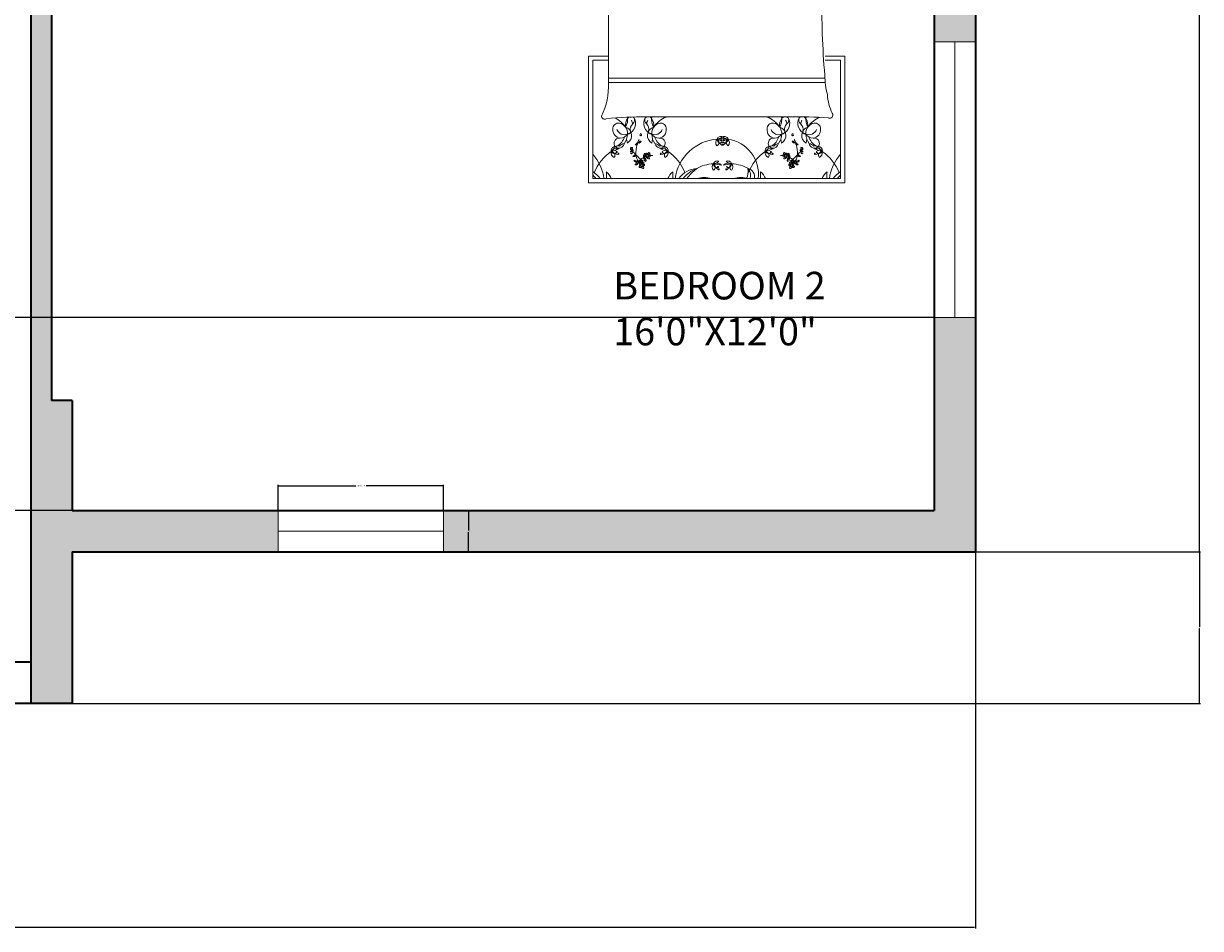
# Model space of a CAD drawing. Units: inches. Extents: x -26 to 13070, y -956 to 6917.
# Tile 3 of 13: x 341 to 597, y -956 to -760. Entities that reach past the tile are written whole.
import ezdxf

# ---------------------------------------------------------------- set-up
doc = ezdxf.new("R2010")
doc.units = ezdxf.units.IN
doc.header["$MEASUREMENT"] = 0
for name, color, linetype, lineweight in [('A-ANNO-DIMS', 2, 'Continuous', 18), ('A-AREA-IDEN', 7, 'Continuous', 18), ('A-FURN', 8, 'Continuous', 13), ('A-GLAZ', 4, 'Continuous', 18), ('A-WALL', 7, 'Continuous', 35), ('A-WALL-PATT', 252, 'Continuous', 13)]:
    doc.layers.add(name, color=color, linetype=linetype, lineweight=lineweight)
doc.styles.get("Standard").update_dxf_attribs({"font": 'arial.ttf'})
doc.dimstyles.get("Standard").update_dxf_attribs({"dimtxt": 0.18, "dimasz": 0.18, "dimexe": 0.18, "dimexo": 0.0625, "dimgap": 0.09, "dimtad": 0, "dimtih": 1, "dimtoh": 1, "dimdec": 0, "dimzin": 0, "dimdsep": 46, "dimlunit": 3, "dimtxsty": 'Standard', "dimcen": 0.09, "dimadec": 0, "dimazin": 0, "dimtfac": 1, "dimtdec": 0, "dimtofl": 0, "dimtmove": 0, "dimatfit": 3, "dimfxl": 1, "dimtolj": 1, "dimtzin": 0, "dimarcsym": 0})

# ---------------------------------------------------------------- blocks, each defined once
blk = doc.blocks.new('BED-DOUBLE-NIGHTSTANDS')
for p, q in [((0, 65), (76.43, 65)), ((15.29, 65), (15.29, 44.02)), ((61.14, 64.02), (15.29, 64.02)), ((7.64, 53.64), (7.64, 63.62)), ((68.79, 53.64), (68.79, 63.62)), ((12.64, 58.63), (2.65, 58.63)), ((63.79, 58.63), (73.78, 58.63)), ((15.29, 52.92), (61.14, 52.92)), ((25.9, 50.65), (34.24, 52.92)), ((36.28, 52.92), (32.09, 47.09)), ((20.33, 48.64), (25.9, 50.65)), ((60.91, 48.96), (33.16, 48.57)), ((60.94, 49.74), (33.73, 49.36)), ((14.6, 43.22), (17.39, 46.47)), ((17.39, 46.47), (20.33, 48.64)), ((32.09, 47.09), (30.39, 42.6)), ((60.87, 46.55), (31.85, 46.44)), ((60.87, 45.77), (31.55, 45.65)), ((15.22, 42.6), (14.6, 43.22)), ((18.32, 42.91), (15.22, 42.6)), ((22.19, 42.6), (18.32, 42.91)), ((25.59, 42.14), (22.19, 42.6)), ((27.6, 41.21), (25.59, 42.14)), ((30.08, 40.59), (27.6, 41.21)), ((30.39, 42.6), (30.08, 40.59)), ((10.09, 27.53), (14.41, 27.53)), ((10.09, 0), (10.09, 27.53)), ((14.41, 26.65), (10.97, 26.65)), ((10.97, 26.65), (10.97, 0.89)), ((64.92, 26.65), (61.55, 26.65)), ((61.57, 27.53), (65.81, 27.53)), ((64.92, 0.89), (64.92, 26.65)), ((65.81, 27.53), (65.81, 0)), ((61.56, 21.81), (14.4, 21.81)), ((61.49, 22.77), (14.41, 22.77)), ((53.73, 14.3), (22.7, 14.3)), ((18.51, 8.63), (18.34, 9.5)), ((23.85, 8.63), (24.02, 9.5)), ((52.05, 8.63), (51.88, 9.5)), ((57.39, 8.63), (57.56, 9.5)), ((10.97, 0.89), (64.92, 0.89)), ((65.81, 0), (10.09, 0))]:
    blk.add_line(p, q)
for points in [[(15.29, 52.26), (0, 52.26), (0, 65)], [(61.14, 65), (61.14, 52.26), (76.43, 52.26), (76.43, 65)], [(7.64, 58.63), (8.53, 60.17)], [(68.79, 58.63), (67.89, 60.17)], [(7.64, 58.63), (8.53, 57.08)], [(68.79, 58.63), (67.89, 57.08)]]:
    blk.add_lwpolyline(points)
for points in [[(19.68, 63.09, 0.074897), (19.77, 58.1, -0.472817)], [(37.86, 57.82, 0.14099), (38.01, 62.91, 0.235245)], [(41.12, 57.82, -0.14099), (40.97, 62.91, -0.235245)], [(56.75, 63.09, -0.074897), (56.66, 58.1, 0.472817)], [(14.44, 36.22, 0.001242), (14.4, 21.72, -0.127202), (12.87, 14.5)], [(61.47, 23.37, 0.056112), (62.02, 19.16, 0.095341), (63.1, 15.11)]]:
    blk.add_lwpolyline(points, format="xyb")
for centre, radius in [((7.64, 58.63), 3.57), ((68.79, 58.63), 3.57), ((7.64, 58.63), 1.78), ((68.79, 58.63), 1.78), ((22.92, 5.86), 0.195), ((52.98, 5.86), 0.195), ((21.65, 3.81), 0.195), ((54.25, 3.81), 0.195)]:
    blk.add_circle(centre, radius)
for centre, radius, start, end in [((61.8, 790.45), 728.57, 266.68521, 267.14978), ((30.15, 35.44), 27.72, 82.2196, 99.497), ((36, 49.44), 13.62, 81.5249, 103.96), ((42.02, 59.28), 3.78, 63.3437, 106.1026), ((47.68, 49.72), 13.44, 76.3427, 101.1841), ((14.63, 790.45), 728.57, 272.85022, 273.31479), ((29.41, 56.1), 9.85, 155.1316, 191.7583), ((47.02, 56.1), 9.85, 348.2417, 24.8684), ((28.85, 55.27), 9.36, 354.0129, 15.8293), ((50.13, 55.27), 9.36, 164.1707, 185.9871), ((22.4, 63.99), 10.24, 255.1039, 281.0369), ((27.79, 71.27), 17.76, 258.0397, 289.2615), ((34.99, 67.39), 13.48, 259.8617, 283.6238), ((42.53, 57.96), 4.05, 245.0183, 288.5407), ((49.61, 63.23), 9.73, 243.8761, 286.1746), ((54.03, 63.99), 10.24, 258.9631, 284.8961), ((198.16, 43.58), 137.33, 176.1, 180.9282), ((-55.48, 41.32), 70.1, 355.8294, 1.553), ((15.91, 70.29), 28.85, 267.4519, 281.3392), ((22.8, 35.91), 6.22, 66.2616, 101.3392), ((35.39, 69.47), 29.64, 250.1194, 259.3383), ((239.96, 38.59), 179.14, 179.1145, 184.8735), ((29.91, 40.53), 0.184, 268.8623, 19.7536), ((13.58, 14.54), 0.705, 183.98, 297.3412), ((21.79, -65.25), 79.56, 89.3433, 95.6887), ((16.65, 11.7), 1.29, 84.4856, 181.0538), ((13.28, 8.92), 5.78, 33.6671, 63.2997), ((16.25, 10.75), 2.3, 355.2933, 76.921), ((21.03, 12.36), 2.95, 145.785, 184.7304), ((15.4, 13.74), 3.17, 328.8218, 9.1554), ((19.32, 13.46), 0.92, 120.0293, 142.325), ((17.85, 12.92), 2.44, 289.2822, 29.1751), ((17.48, 12.48), 2.2, 7.436, 29.9149), ((18.93, 13.64), 1.14, 311.5653, 23.8354), ((19.32, 13.46), 0.92, 44.4517, 63.558), ((24.5, 12.92), 2.44, 150.8249, 250.7178), ((23.42, 13.64), 1.14, 156.1646, 228.4347), ((23.03, 13.46), 0.92, 113.229, 135.5483), ((24.87, 12.48), 2.2, 150.0851, 172.564), ((23.03, 13.46), 0.92, 37.675, 66.7144), ((21.32, 12.36), 2.95, 355.2696, 34.215), ((26.95, 13.74), 3.17, 169.7133, 211.1782), ((26.1, 10.75), 2.3, 103.079, 184.7067), ((29.07, 8.92), 5.78, 111.4941, 146.3329), ((25.7, 11.7), 1.29, 358.9462, 95.5144), ((50.19, 11.7), 1.29, 84.4856, 181.0538), ((46.82, 8.92), 5.78, 33.6671, 68.5059), ((49.8, 10.75), 2.3, 355.2933, 76.921), ((54.57, 12.36), 2.95, 145.785, 184.7304), ((48.94, 13.74), 3.17, 328.8218, 10.2867), ((52.87, 13.46), 0.92, 113.2856, 142.325), ((51.4, 12.92), 2.44, 289.2822, 29.1751), ((51.03, 12.48), 2.2, 7.436, 29.9149), ((52.87, 13.46), 0.92, 44.4517, 66.7144), ((52.48, 13.64), 1.14, 311.5653, 23.8354), ((56.07, -60.03), 74.37, 85.2402, 91.8035), ((58.04, 12.92), 2.44, 150.8249, 250.7178), ((56.96, 13.64), 1.14, 156.1646, 228.4347), ((56.57, 13.46), 0.92, 106.6343, 135.5483), ((58.41, 12.48), 2.2, 150.0851, 172.564), ((56.57, 13.46), 0.92, 37.675, 72.5814), ((54.87, 12.36), 2.95, 355.2696, 34.215), ((60.5, 13.74), 3.17, 169.249, 211.1782), ((59.64, 10.75), 2.3, 103.079, 184.7067), ((62.62, 8.92), 5.78, 113.6453, 146.3329), ((59.25, 11.7), 1.29, 358.9462, 95.5144), ((62.52, 14.72), 0.697, 246.5219, 33.8264), ((17.18, 11.52), 1.83, 174.9449, 262.8857), ((17.9, 12.21), 1.77, 201.5819, 291.4221), ((16.86, 11.92), 2.22, 272.3591, 324.0401), ((14.45, 10.81), 4.1, 326.2883, 356.5076), ((17.56, 10.28), 1.9, 299.9085, 73.1337), ((21.03, 12.36), 2.95, 212.7011, 216.3445), ((18.76, 11.08), 0.474, 257.3041, 15.1471), ((20.73, 11.61), 1.57, 131.5653, 195.1471), ((21.4, 10.36), 0.147, 102.7051, 280.4384), ((21.38, 10.45), 0.24, 280.4384, 100.4136), ((21.62, 11.61), 1.57, 344.8529, 48.4347), ((24.79, 10.28), 1.9, 106.8663, 240.0915), ((23.59, 11.08), 0.474, 164.8529, 282.6959), ((21.32, 12.36), 2.95, 323.6555, 327.2989), ((25.49, 11.92), 2.22, 215.9599, 267.6409), ((24.46, 12.21), 1.77, 248.5779, 338.4181), ((27.9, 10.81), 4.1, 183.4924, 213.7117), ((25.17, 11.52), 1.83, 277.1143, 5.0551), ((50.72, 11.52), 1.83, 174.9449, 262.8857), ((51.44, 12.21), 1.77, 201.5819, 291.4221), ((50.4, 11.92), 2.22, 272.3591, 324.0401), ((47.99, 10.81), 4.1, 326.2883, 356.5076), ((51.1, 10.28), 1.9, 299.9085, 73.1337), ((54.57, 12.36), 2.95, 212.7011, 216.3445), ((52.3, 11.08), 0.474, 257.3041, 15.1471), ((54.28, 11.61), 1.57, 131.5653, 195.1471), ((54.52, 10.45), 0.24, 79.5864, 259.5616), ((54.5, 10.36), 0.147, 259.5616, 77.2949), ((55.16, 11.61), 1.57, 344.8529, 48.4347), ((58.34, 10.28), 1.9, 106.8663, 240.0915), ((57.13, 11.08), 0.474, 164.8529, 282.6959), ((54.87, 12.36), 2.95, 323.6555, 327.2989), ((59.04, 11.92), 2.22, 215.9599, 267.6409), ((58, 12.21), 1.77, 248.5779, 338.4181), ((61.45, 10.81), 4.1, 183.4924, 213.7117), ((58.72, 11.52), 1.83, 277.1143, 5.0551), ((15.79, 6.99), 0.827, 92.9516, 193.728), ((14.09, 8.25), 1.7, 301.3827, 345.2969), ((16.76, 8.57), 1.15, 80.264, 250.8688), ((16.52, 7.33), 0.703, 63.9755, 143.2681), ((14.48, 11.1), 3.61, 301.2614, 341.7045), ((16.48, 8.92), 1.43, 265.969, 344.3045), ((18.02, 7.01), 1.53, 96.1662, 141.5825), ((19.47, 7.55), 0.15, 345.2356, 144.9248), ((20.55, 8.08), 0.401, 101.3256, 154.4621), ((19.97, 9.45), 1.21, 280.2588, 300.656), ((20.25, 10.41), 2.16, 268.3264, 277.1302), ((26.69, 6.51), 6.33, 163.5842, 183.8277), ((19.71, 9.44), 1.23, 308.2101, 316.3071), ((20.47, 8.64), 0.367, 278.3432, 4.2869), ((20.26, 8.96), 0.641, 300.656, 332.6341), ((20.74, 8.53), 0.156, 55.7657, 157.4417), ((26.69, 6.51), 6.33, 153.0032, 159.8941), ((20.99, 8.68), 0.156, 84.3784, 186.0543), ((20.84, 9.3), 0.641, 269.1859, 301.164), ((21.03, 8.97), 0.367, 237.5332, 323.4768), ((20.67, 10.02), 1.23, 285.5129, 293.6099), ((20.55, 9.79), 1.21, 301.164, 321.5612), ((21.48, 8.64), 0.401, 87.3579, 140.4944), ((19.56, 10), 2.16, 324.6898, 333.4936), ((27.87, 11.1), 3.61, 198.2955, 238.7386), ((24.33, 7.01), 1.53, 38.4175, 83.8338), ((25.87, 8.92), 1.43, 195.6955, 274.031), ((25.59, 8.57), 1.15, 289.1312, 99.736), ((25.83, 7.33), 0.703, 36.7319, 116.0245), ((26.57, 6.99), 0.827, 346.272, 87.0484), ((28.26, 8.25), 1.7, 194.7031, 238.6173), ((38.81, -0.46), 9.98, 94.4623, 172.255), ((38.85, 8.75), 1.11, 137.7873, 219.1145), ((37.6, 8.78), 0.834, 298.5391, 58.3627), ((38.83, 9.26), 0.827, 63.0274, 163.8037), ((37.99, 11.2), 1.7, 271.4585, 315.3727), ((38.68, 8.05), 1.58, 45.5411, 114.3101), ((40.12, 16.15), 6.98, 252.593, 267.2582), ((38.85, 9.46), 0.816, 177.7585, 283.852), ((40.42, 10.31), 2.52, 198.9159, 238.011), ((39.76, 8.05), 1.58, 65.6899, 134.4589), ((38.32, 16.15), 6.98, 272.7418, 287.407), ((39.02, 8.77), 0.108, 283.852, 219.9245), ((39.15, 8.27), 0.124, 238.011, 71.5592), ((39.17, 8.33), 0.0602, 71.5592, 188.0167), ((39.29, 8.27), 0.124, 108.4408, 301.989), ((39.62, 9.26), 0.827, 16.1963, 116.9726), ((40.45, 11.2), 1.7, 224.6273, 268.5415), ((39.27, 8.33), 0.0602, 351.9833, 108.4408), ((39.42, 8.81), 0.0651, 320.1909, 256.0209), ((38.02, 10.31), 2.52, 301.989, 341.0841), ((39.6, 9.46), 0.816, 256.148, 2.2415), ((40.85, 8.78), 0.834, 121.6373, 241.4609), ((39.59, 8.75), 1.11, 320.8855, 42.2127), ((39.31, 1.85), 7.72, 352.8636, 81.8197), ((49.33, 6.99), 0.827, 92.9516, 193.728), ((47.64, 8.25), 1.7, 301.3827, 345.2969), ((50.3, 8.57), 1.15, 80.264, 250.8688), ((50.06, 7.33), 0.703, 63.9755, 143.2681), ((48.03, 11.1), 3.61, 301.2614, 341.7045), ((50.03, 8.92), 1.43, 265.969, 344.3045), ((51.57, 7.01), 1.53, 96.1662, 141.5825), ((55.35, 9.79), 1.21, 218.4388, 238.836), ((54.42, 8.64), 0.401, 39.5056, 92.6421), ((56.33, 10), 2.16, 206.5064, 215.3102), ((54.87, 8.97), 0.367, 216.5232, 302.4668), ((55.05, 9.3), 0.641, 238.836, 270.8141), ((55.22, 10.02), 1.23, 246.3901, 254.4871), ((49.2, 6.51), 6.33, 20.1059, 26.9968), ((54.91, 8.68), 0.156, 353.9457, 95.6216), ((55.15, 8.53), 0.156, 22.5583, 124.2343), ((55.43, 8.64), 0.367, 175.7131, 261.6568), ((55.63, 8.96), 0.641, 207.3659, 239.344), ((49.2, 6.51), 6.33, 356.1723, 16.4158), ((56.18, 9.44), 1.23, 223.6929, 231.7899), ((55.92, 9.45), 1.21, 239.344, 259.7412), ((55.64, 10.41), 2.16, 262.8698, 271.6736), ((55.34, 8.08), 0.401, 25.5379, 78.6744), ((56.42, 7.55), 0.15, 35.0752, 194.7644), ((61.41, 11.1), 3.61, 198.2955, 238.7386), ((59.41, 8.92), 1.43, 195.6955, 274.031), ((57.87, 7.01), 1.53, 38.4175, 83.8338), ((59.14, 8.57), 1.15, 289.1312, 99.736), ((59.37, 7.33), 0.703, 36.7319, 116.0245), ((61.8, 8.25), 1.7, 194.7031, 238.6173), ((60.11, 6.99), 0.827, 346.272, 87.0484), ((3.54, -0.46), 9.98, 7.745, 41.8856), ((20.62, -1.45), 9.98, 124.3865, 158.5908), ((16.06, 6.55), 1.11, 167.7115, 249.0387), ((16.26, 5.87), 1.58, 75.4653, 144.2343), ((13.47, 13.61), 6.98, 282.5173, 297.1824), ((14.96, 5.96), 0.834, 328.4633, 88.2869), ((16.64, 8.69), 2.52, 228.8402, 267.9352), ((15.7, 7.17), 0.816, 207.6827, 313.7762), ((16.19, 6.66), 0.108, 313.7762, 249.7183), ((16.54, 6.35), 0.0602, 101.4834, 217.9409), ((16.56, 6.29), 0.124, 267.9352, 101.4834), ((19.42, 7.32), 0.325, 101.5637, 142.6358), ((19.15, 7.02), 0.195, 273.2768, 86.7232), ((19.41, 6.66), 0.321, 217.7621, 259.0403), ((19.37, 7.21), 0.186, 91.1081, 181.8675), ((19.76, 7.09), 0.591, 203.4276, 227.6104), ((19.57, 6.83), 0.402, 80.3487, 133.6538), ((19.5, 7.16), 0.318, 229.7889, 317.6792), ((19.16, 7.58), 0.468, 288.7263, 352.5032), ((19.14, 6.49), 0.452, 355.053, 68.3618), ((19.5, 6.41), 0.637, 83.0852, 105.7171), ((19.44, 6.46), 0.149, 232.4737, 355.053), ((15.08, 1.13), 7.26, 43.1541, 52.0459), ((19.61, 7.06), 0.168, 317.6792, 80.3487), ((20.1, 5.51), 0.401, 101.3256, 154.4621), ((19.52, 6.87), 1.21, 280.2588, 300.656), ((19.8, 7.84), 2.16, 268.3264, 277.1302), ((19.26, 6.87), 1.23, 308.2101, 316.3071), ((20.01, 6.06), 0.367, 278.3432, 4.2869), ((19.81, 6.39), 0.641, 300.656, 332.6341), ((20.29, 5.96), 0.156, 55.7657, 157.4417), ((23.54, 6.35), 3.17, 184.756, 209.2041), ((28.11, 13.11), 10.44, 222.2412, 232.1744), ((23.87, 2.14), 3.81, 120.544, 139.818), ((21.43, 6.15), 0.887, 304.5369, 16.3699), ((21.9, 5.96), 0.539, 272.8499, 356.1226), ((21.52, 5.75), 0.522, 321.7607, 7.9252), ((21.63, 5), 0.522, 8.7227, 54.8872), ((21.66, 4.58), 0.887, 0.278, 72.111), ((22.66, 5.9), 0.628, 127.3105, 187.9252), ((22.06, 4.9), 0.539, 20.5253, 88.5375), ((21.8, 5.98), 0.645, 355.0106, 41.658), ((22.51, 5.5), 0.193, 148.0499, 225.6268), ((23.87, 2.14), 3.81, 113.0501, 113.8477), ((22.87, 5.28), 0.614, 104.7558, 148.0499), ((22.52, 5.72), 0.384, 247.4086, 351.4386), ((22.71, 6.14), 0.265, 126.1046, 271.4281), ((22.68, 6.21), 0.191, 353.7526, 131.7054), ((22.63, 5.7), 0.129, 262.906, 7.132), ((22.5, 5.98), 0.268, 0.0645, 61.1507), ((22.56, 6.21), 0.306, 311.8413, 355.7877), ((23.19, 5.5), 0.321, 151.2196, 259.0403), ((23.19, 6.17), 0.325, 101.5637, 176.365), ((23.15, 6.05), 0.186, 91.1081, 181.8675), ((23.53, 5.93), 0.591, 203.4276, 227.6104), ((23.35, 5.67), 0.402, 80.3487, 133.6538), ((23.27, 6.01), 0.318, 229.7889, 317.6792), ((22.93, 6.42), 0.468, 288.7263, 352.5032), ((22.91, 5.33), 0.452, 355.053, 68.3618), ((23.27, 5.26), 0.637, 83.0852, 105.7171), ((23.25, 6.4), 0.15, 345.2356, 144.9248), ((23.22, 5.31), 0.149, 232.4737, 355.053), ((23.38, 5.91), 0.168, 317.6792, 80.3487), ((23.87, 2.14), 3.81, 87.1071, 94.7585), ((25.8, 6.29), 0.124, 78.5166, 272.0648), ((26.09, 5.87), 1.58, 35.7657, 104.5347), ((28.88, 13.61), 6.98, 242.8176, 257.4827), ((25.71, 8.69), 2.52, 272.0648, 311.1598), ((25.81, 6.35), 0.0602, 322.0591, 78.5166), ((26.65, 7.17), 0.816, 226.2238, 332.3173), ((26.17, 6.7), 0.0651, 290.2667, 226.2271), ((27.4, 5.96), 0.834, 91.7131, 211.5367), ((26.29, 6.55), 1.11, 290.9613, 12.2885), ((21.73, -1.45), 9.98, 21.4092, 55.6135), ((54.16, -1.45), 9.98, 124.3865, 158.5908), ((49.61, 6.55), 1.11, 167.7115, 249.0387), ((49.81, 5.87), 1.58, 75.4653, 144.2343), ((47.01, 13.61), 6.98, 282.5173, 297.1824), ((49.25, 7.17), 0.816, 207.6827, 313.7762), ((50.19, 8.69), 2.52, 228.8402, 267.9352), ((48.5, 5.96), 0.834, 328.4633, 88.2869), ((49.74, 6.66), 0.108, 313.7762, 249.7183), ((50.09, 6.35), 0.0602, 101.4834, 217.9409), ((50.1, 6.29), 0.124, 267.9352, 101.4834), ((52.03, 2.14), 3.81, 85.2415, 92.8929), ((52.51, 5.91), 0.168, 99.6513, 222.3208), ((52.62, 6.01), 0.318, 222.3208, 310.2111), ((52.55, 5.67), 0.402, 46.3462, 99.6513), ((52.65, 6.4), 0.15, 35.0752, 194.7644), ((52.97, 6.42), 0.468, 187.4968, 251.2737), ((52.98, 5.33), 0.452, 111.6382, 184.947), ((52.68, 5.31), 0.149, 184.947, 307.5263), ((52.63, 5.26), 0.637, 74.2829, 96.9148), ((52.75, 6.05), 0.186, 358.1325, 88.8919), ((52.36, 5.93), 0.591, 312.3896, 336.5724), ((52.71, 6.17), 0.325, 3.635, 78.4363), ((52.71, 5.5), 0.321, 280.9597, 28.7804), ((53.37, 5.72), 0.384, 188.5614, 292.5914), ((53.22, 6.21), 0.191, 48.2946, 186.2474), ((53.34, 6.21), 0.306, 184.2123, 228.1587), ((53.4, 5.98), 0.268, 118.8493, 179.9355), ((53.26, 5.7), 0.129, 172.868, 277.094), ((53.19, 6.14), 0.265, 268.5719, 53.8954), ((53.03, 5.28), 0.614, 31.9501, 75.2442), ((53.84, 4.9), 0.539, 91.4625, 159.4747), ((54.23, 4.58), 0.887, 107.889, 179.722), ((54.1, 5.98), 0.645, 138.342, 184.9894), ((53.99, 5.96), 0.539, 183.8774, 267.1501), ((52.03, 2.14), 3.81, 66.1523, 66.9499), ((53.38, 5.5), 0.193, 314.3732, 31.9501), ((54.47, 6.15), 0.887, 163.6301, 235.4631), ((53.23, 5.9), 0.628, 352.0748, 52.6895), ((54.26, 5), 0.522, 125.1128, 171.2773), ((54.37, 5.75), 0.522, 172.0748, 218.2393), ((52.03, 2.14), 3.81, 40.182, 59.456), ((47.79, 13.11), 10.44, 307.8256, 317.7588), ((52.36, 6.35), 3.17, 330.7959, 355.244), ((60.81, 1.13), 7.26, 127.9541, 136.8459), ((55.61, 5.96), 0.156, 22.5583, 124.2343), ((55.88, 6.06), 0.367, 175.7131, 261.6568), ((56.09, 6.39), 0.641, 207.3659, 239.344), ((56.64, 6.87), 1.23, 223.6929, 231.7899), ((56.38, 6.87), 1.21, 239.344, 259.7412), ((56.1, 7.84), 2.16, 262.8698, 271.6736), ((55.8, 5.51), 0.401, 25.5379, 78.6744), ((56.28, 7.06), 0.168, 99.6513, 222.3208), ((56.4, 7.16), 0.318, 222.3208, 310.2111), ((56.32, 6.83), 0.402, 46.3462, 99.6513), ((56.74, 7.58), 0.468, 187.4968, 251.2737), ((56.76, 6.49), 0.452, 111.6382, 184.947), ((56.45, 6.46), 0.149, 184.947, 307.5263), ((56.4, 6.41), 0.637, 74.2829, 96.9148), ((56.52, 7.21), 0.186, 358.1325, 88.8919), ((56.14, 7.09), 0.591, 312.3896, 336.5724), ((56.48, 7.32), 0.325, 37.3642, 78.4363), ((56.48, 6.66), 0.321, 280.9597, 322.2379), ((56.75, 7.02), 0.195, 93.2768, 266.7232), ((59.34, 6.29), 0.124, 78.5166, 272.0648), ((59.63, 5.87), 1.58, 35.7657, 104.5347), ((62.43, 13.61), 6.98, 242.8176, 257.4827), ((59.25, 8.69), 2.52, 272.0648, 311.1598), ((59.35, 6.35), 0.0602, 322.0591, 78.5166), ((60.19, 7.17), 0.816, 226.2238, 332.3173), ((59.71, 6.7), 0.0651, 290.2667, 226.2271), ((60.94, 5.96), 0.834, 91.7131, 211.5367), ((59.83, 6.55), 1.11, 290.9613, 12.2885), ((55.28, -1.45), 9.98, 21.4092, 55.6135), ((72.35, -0.46), 9.98, 138.1144, 172.255), ((20.23, 4.81), 0.217, 146.8636, 236.9021), ((23.3, 9.6), 5.69, 235.1882, 238.8844), ((20.6, 5.12), 0.588, 199.4799, 267.6828), ((20.54, 4.9), 0.507, 212.8155, 277.3992), ((20.24, 4.56), 0.588, 266.9701, 338.2913), ((17.14, 8.76), 5.69, 302.6784, 306.3746), ((20.39, 4.1), 0.217, 214.3538, 304.3923), ((20.47, 4.92), 0.225, 238.8844, 314.2646), ((20.42, 4.42), 0.507, 280.3057, 17.1958), ((20.38, 4.36), 0.225, 306.3746, 21.7548), ((20.75, 4.51), 0.17, 19.3605, 201.7548), ((20.75, 4.64), 0.17, 311.8703, 134.2646), ((23.94, 3.09), 3.39, 153.7819, 158.2913), ((21.24, 5.41), 0.887, 247.2305, 319.0635), ((20.95, 5.11), 0.522, 264.4544, 310.6188), ((23.54, 6.35), 3.17, 214.0033, 222.4917), ((21.33, 4.9), 0.539, 218.3208, 298.8162), ((21.24, 3.45), 0.193, 148.0499, 225.6268), ((21.6, 3.23), 0.614, 104.7558, 148.0499), ((21.25, 3.66), 0.384, 247.4086, 351.4386), ((21.43, 4.08), 0.265, 126.1046, 271.4281), ((21.4, 4.16), 0.191, 353.7526, 131.7054), ((21.7, 4.23), 0.628, 70.0041, 130.6188), ((21.36, 3.65), 0.129, 262.906, 7.132), ((21.22, 3.93), 0.268, 0.0645, 61.1507), ((21.29, 4.16), 0.306, 311.8413, 355.7877), ((21.29, 5), 0.645, 297.7043, 344.3516), ((21.92, 4.11), 0.325, 101.5637, 176.365), ((21.91, 3.45), 0.321, 151.2196, 259.0403), ((21.87, 4), 0.186, 91.1081, 181.8675), ((22.26, 3.88), 0.591, 203.4276, 227.6104), ((22.07, 3.62), 0.402, 80.3487, 133.6538), ((22, 3.96), 0.318, 229.7889, 317.6792), ((21.66, 4.37), 0.468, 288.7263, 352.5032), ((21.64, 3.28), 0.452, 355.053, 68.3618), ((22, 3.21), 0.637, 83.0852, 105.7171), ((21.97, 4.35), 0.15, 345.2356, 144.9248), ((21.94, 3.26), 0.149, 232.4737, 355.053), ((22.11, 3.85), 0.168, 317.6792, 80.3487), ((22.77, 5.17), 0.628, 188.7227, 249.3375), ((21.96, 4.86), 0.645, 334.9899, 21.6373), ((33.8, -1.8), 4.86, 91.272, 146.5383), ((35.55, -2.7), 6.06, 107.8504, 143.6964), ((38.74, -4.41), 9.02, 124.0123, 144.053), ((38.04, -5.81), 9.98, 94.4623, 117.4146), ((38.09, 3.4), 1.11, 137.7873, 219.1145), ((36.83, 3.44), 0.834, 298.5391, 58.3627), ((38.06, 3.91), 0.827, 63.0274, 163.8037), ((37.22, 5.85), 1.7, 271.4585, 315.3727), ((37.92, 2.71), 1.58, 45.5411, 114.3101), ((39.66, 4.96), 2.52, 198.9159, 238.011), ((39.36, 10.81), 6.98, 252.593, 267.2582), ((38.08, 4.11), 0.816, 177.7585, 283.852), ((38.25, 3.43), 0.108, 283.852, 219.9245), ((38.38, 2.93), 0.124, 238.011, 71.5592), ((38.4, 2.99), 0.0602, 71.5592, 188.0167), ((40.53, 2.71), 1.58, 65.6899, 134.4589), ((39.09, 10.81), 6.98, 272.7418, 287.407), ((40.06, 2.93), 0.124, 108.4408, 301.989), ((40.38, 3.91), 0.827, 16.1963, 116.9726), ((41.22, 5.85), 1.7, 224.6273, 268.5415), ((40.04, 2.99), 0.0602, 351.9833, 108.4408), ((40.18, 3.47), 0.0651, 320.1909, 256.0209), ((38.79, 4.96), 2.52, 301.989, 341.0841), ((40.36, 4.11), 0.816, 256.148, 2.2415), ((41.61, 3.44), 0.834, 121.6373, 241.4609), ((40.36, 3.4), 1.11, 320.8855, 42.2127), ((40.4, -5.81), 9.98, 62.5854, 85.5377), ((40.31, 2.55), 4.47, 338.117, 6.6195), ((44.41, 1.31), 1.79, 346.3898, 79.0739), ((43.06, 1.55), 2.27, 342.8609, 41.9049), ((53.93, 4.86), 0.645, 158.3627, 205.0101), ((53.13, 5.17), 0.628, 290.6625, 351.2773), ((53.78, 3.85), 0.168, 99.6513, 222.3208), ((53.9, 3.96), 0.318, 222.3208, 310.2111), ((53.82, 3.62), 0.402, 46.3462, 99.6513), ((53.92, 4.35), 0.15, 35.0752, 194.7644), ((54.24, 4.37), 0.468, 187.4968, 251.2737), ((54.26, 3.28), 0.452, 111.6382, 184.947), ((53.95, 3.26), 0.149, 184.947, 307.5263), ((53.9, 3.21), 0.637, 74.2829, 96.9148), ((54.2, 4.23), 0.628, 49.3812, 109.9959), ((54.65, 5.41), 0.887, 220.9365, 292.7695), ((54.6, 5), 0.645, 195.6484, 242.2957), ((54.02, 4), 0.186, 358.1325, 88.8919), ((53.64, 3.88), 0.591, 312.3896, 336.5724), ((53.98, 4.11), 0.325, 3.635, 78.4363), ((53.98, 3.45), 0.321, 280.9597, 28.7804), ((54.64, 3.66), 0.384, 188.5614, 292.5914), ((54.56, 4.9), 0.539, 241.1838, 321.6792), ((54.49, 4.16), 0.191, 48.2946, 186.2474), ((54.61, 4.16), 0.306, 184.2123, 228.1587), ((54.67, 3.93), 0.268, 118.8493, 179.9355), ((54.54, 3.65), 0.129, 172.868, 277.094), ((54.46, 4.08), 0.265, 268.5719, 53.8954), ((54.3, 3.23), 0.614, 31.9501, 75.2442), ((54.95, 5.11), 0.522, 229.3812, 275.5456), ((52.36, 6.35), 3.17, 317.5083, 325.9967), ((54.66, 3.45), 0.193, 314.3732, 31.9501), ((55.47, 4.42), 0.507, 162.8042, 259.6943), ((55.15, 4.64), 0.17, 45.7354, 228.1297), ((55.15, 4.51), 0.17, 338.2452, 160.6395), ((51.96, 3.09), 3.39, 21.7087, 26.2181), ((55.65, 4.56), 0.588, 201.7087, 273.0299), ((55.42, 4.92), 0.225, 225.7354, 301.1156), ((55.36, 4.9), 0.507, 262.6008, 327.1845), ((55.51, 4.36), 0.225, 158.2452, 233.6254), ((55.29, 5.12), 0.588, 272.3172, 340.5201), ((58.75, 8.76), 5.69, 233.6254, 237.3216), ((55.5, 4.1), 0.217, 235.6077, 325.6462), ((52.6, 9.6), 5.69, 301.1156, 304.8118), ((55.66, 4.81), 0.217, 303.0979, 33.1364), ((8.55, -1.8), 4.86, 33.4617, 60.1116), ((6.8, -2.7), 6.06, 36.3036, 46.4814), ((11.27, -0.67), 4.06, 22.5547, 48.9546), ((0.16, 1.51), 13.81, 357.4081, 3.6519), ((31.08, -0.67), 4.06, 131.0454, 157.4453), ((42.19, 1.51), 13.81, 176.3481, 182.5919), ((35.25, -4.36), 5.49, 73.5431, 107.0202), ((37.43, -7.19), 8.12, 94.3787, 95.6357), ((41.7, -12.75), 14.5, 109.7217, 109.9028), ((43.19, -4.36), 5.49, 72.9798, 106.4569), ((41.02, -7.19), 8.12, 84.3643, 85.6213), ((36.74, -12.75), 14.5, 70.0972, 70.2783), ((33.7, 1.51), 13.81, 357.4081, 3.6519), ((44.82, -0.67), 4.06, 22.5547, 48.9546), ((64.62, -0.67), 4.06, 131.0454, 157.4453), ((75.74, 1.51), 13.81, 176.3481, 182.5919), ((67.35, -1.8), 4.86, 119.8884, 146.5383), ((69.1, -2.7), 6.06, 133.5186, 143.6964)]:
    blk.add_arc(centre, radius, start, end)
blk = doc.blocks.new('WIN-36')
for p, q in [((0, 36), (0, 0)), ((9, 36), (0, 36)), ((4.5, 36), (4.5, 0)), ((9, 0), (9, 36)), ((0, 0), (9, 0))]:
    blk.add_line(p, q)
blk = doc.blocks.new('WIN-60')
for p, q in [((0, 0), (0, 60)), ((0, 60), (9, 60)), ((4.5, 0), (4.5, 60)), ((9, 60), (9, 0)), ((9, 0), (0, 0))]:
    blk.add_line(p, q)
blk = doc.blocks.new('*D18')
at = {"layer": 'A-ANNO-DIMS', "color": 0, "lineweight": -2, "transparency": 16777216}
for p, q in [((395.95, -865.48), (395.95, -859.96)), ((396.13, -860.14), (412.83, -860.14)), ((431.77, -860.14), (415.07, -860.14)), ((431.95, -865.48), (431.95, -859.96))]:
    blk.add_line(p, q, dxfattribs=at)
at = {"layer": 'A-ANNO-DIMS', "color": 0, "transparency": 16777216}
for points in [[(396.13, -860.11), (396.13, -860.17), (395.95, -860.14)], [(431.77, -860.11), (431.77, -860.17), (431.95, -860.14)]]:
    blk.add_solid(points, dxfattribs=at)
at = {"layer": 'Defpoints', "color": 0, "transparency": 16777216}
for p in [(395.95, -860.14), (395.95, -865.54), (431.95, -865.54)]:
    blk.add_point(p, dxfattribs=at)
at = {"layer": 'A-ANNO-DIMS', "color": 0, "transparency": 16777216, "insert": (413.95, -860.14), "char_height": 0.18, "attachment_point": 5}
blk.add_mtext('\\A1;WINDOW 36 TYP.', dxfattribs=at)
blk = doc.blocks.new('*D19')
at = {"layer": 'A-ANNO-DIMS', "color": 0, "lineweight": -2, "transparency": 16777216}
for p, q in [((432.01, -865.54), (437.53, -865.54)), ((437.35, -865.72), (437.35, -869.86)), ((437.35, -874.36), (437.35, -870.22)), ((432.01, -874.54), (437.53, -874.54))]:
    blk.add_line(p, q, dxfattribs=at)
at = {"layer": 'A-ANNO-DIMS', "color": 0, "transparency": 16777216}
for points in [[(437.32, -865.72), (437.38, -865.72), (437.35, -865.54)], [(437.32, -874.36), (437.38, -874.36), (437.35, -874.54)]]:
    blk.add_solid(points, dxfattribs=at)
at = {"layer": 'Defpoints', "color": 0, "transparency": 16777216}
for p in [(431.95, -865.54), (437.35, -865.54), (431.95, -874.54)]:
    blk.add_point(p, dxfattribs=at)
at = {"layer": 'A-ANNO-DIMS', "color": 0, "transparency": 16777216, "insert": (437.35, -870.04), "char_height": 0.18, "attachment_point": 5}
blk.add_mtext('\\A1;9 TYP.', dxfattribs=at)
blk = doc.blocks.new('*D40')
at = {"layer": 'A-ANNO-DIMS', "color": 0, "lineweight": -2, "transparency": 16777216}
for p, q in [((22.64, -874.6), (22.64, -956.47)), ((547.64, -874.6), (547.64, -956.47)), ((22.82, -956.29), (284.85, -956.29)), ((547.46, -956.29), (285.43, -956.29))]:
    blk.add_line(p, q, dxfattribs=at)
at = {"layer": 'A-ANNO-DIMS', "color": 0, "transparency": 16777216}
for points in [[(22.82, -956.26), (22.82, -956.32), (22.64, -956.29)], [(547.46, -956.26), (547.46, -956.32), (547.64, -956.29)]]:
    blk.add_solid(points, dxfattribs=at)
at = {"layer": 'Defpoints', "color": 0, "transparency": 16777216}
for p in [(22.64, -874.54), (547.64, -874.54), (547.64, -956.29)]:
    blk.add_point(p, dxfattribs=at)
at = {"layer": 'A-ANNO-DIMS', "color": 0, "transparency": 16777216, "insert": (285.14, -956.29), "char_height": 0.18, "attachment_point": 5}
blk.add_mtext('\\A1;525', dxfattribs=at)
blk = doc.blocks.new('*D46')
at = {"layer": 'A-ANNO-DIMS', "color": 0, "lineweight": -2, "transparency": 16777216}
for p, q in [((538.7, -457.54), (596.57, -457.54)), ((596.39, -457.72), (596.39, -665.86)), ((596.39, -874.36), (596.39, -666.22)), ((547.7, -874.54), (596.57, -874.54))]:
    blk.add_line(p, q, dxfattribs=at)
at = {"layer": 'A-ANNO-DIMS', "color": 0, "transparency": 16777216}
for points in [[(596.36, -457.72), (596.42, -457.72), (596.39, -457.54)], [(596.36, -874.36), (596.42, -874.36), (596.39, -874.54)]]:
    blk.add_solid(points, dxfattribs=at)
at = {"layer": 'Defpoints', "color": 0, "transparency": 16777216}
for p in [(538.64, -457.54), (596.39, -457.54), (547.64, -874.54)]:
    blk.add_point(p, dxfattribs=at)
at = {"layer": 'A-ANNO-DIMS', "color": 0, "transparency": 16777216, "insert": (596.39, -666.04), "char_height": 0.18, "attachment_point": 5}
blk.add_mtext('\\A1;417', dxfattribs=at)
blk = doc.blocks.new('*D48')
at = {"layer": 'A-ANNO-DIMS', "color": 0, "lineweight": -2, "transparency": 16777216}
for p, q in [((547.7, -874.54), (596.57, -874.54)), ((596.39, -874.72), (596.39, -890.86)), ((596.39, -907.36), (596.39, -891.22)), ((351.2, -907.54), (596.57, -907.54))]:
    blk.add_line(p, q, dxfattribs=at)
at = {"layer": 'A-ANNO-DIMS', "color": 0, "transparency": 16777216}
for points in [[(596.36, -874.72), (596.42, -874.72), (596.39, -874.54)], [(596.36, -907.36), (596.42, -907.36), (596.39, -907.54)]]:
    blk.add_solid(points, dxfattribs=at)
at = {"layer": 'Defpoints', "color": 0, "transparency": 16777216}
for p in [(547.64, -874.54), (596.39, -874.54), (351.14, -907.54)]:
    blk.add_point(p, dxfattribs=at)
at = {"layer": 'A-ANNO-DIMS', "color": 0, "transparency": 16777216, "insert": (596.39, -891.04), "char_height": 0.18, "attachment_point": 5}
blk.add_mtext('\\A1;33', dxfattribs=at)
blk = doc.blocks.new('*D59')
at = {"layer": 'A-ANNO-DIMS', "color": 0, "lineweight": -2, "transparency": 16777216}
for p, q in [((538.58, -823.54), (-26.29, -823.54)), ((-26.11, -823.72), (-26.11, -844.36)), ((-26.11, -865.36), (-26.11, -844.72)), ((538.58, -865.54), (-26.29, -865.54))]:
    blk.add_line(p, q, dxfattribs=at)
at = {"layer": 'A-ANNO-DIMS', "color": 0, "transparency": 16777216}
for points in [[(-26.14, -823.72), (-26.08, -823.72), (-26.11, -823.54)], [(-26.14, -865.36), (-26.08, -865.36), (-26.11, -865.54)]]:
    blk.add_solid(points, dxfattribs=at)
at = {"layer": 'Defpoints', "color": 0, "transparency": 16777216}
for p in [(-26.11, -823.54), (538.64, -823.54), (538.64, -865.54)]:
    blk.add_point(p, dxfattribs=at)
at = {"layer": 'A-ANNO-DIMS', "color": 0, "transparency": 16777216, "insert": (-26.11, -844.54), "char_height": 0.18, "attachment_point": 5}
blk.add_mtext('\\A1;42', dxfattribs=at)

msp = doc.modelspace()

# ---------------------------------------------------------------- hatches: boundary and pattern name
at = {"layer": 'A-WALL-PATT'}
h = msp.add_hatch(color=256, dxfattribs=at)
h.dxf.hatch_style = 1
h.paths.add_polyline_path([(223.641, 10.458), (214.641, 10.458), (22.641, 10.458), (22.641, -171.042), (31.641, -171.042), (31.641, -135.042), (205.641, -135.042), (205.641, -241.042), (210.141, -241.042), (210.141, -130.542), (94.641, -130.542), (94.641, -76.542), (85.641, -76.542), (85.641, -126.042), (27.141, -126.042), (27.141, 5.958), (85.641, 5.958), (85.641, -52.542), (94.641, -52.542), (94.641, 1.458), (214.641, 1.458), (214.641, -16.542), (223.641, -16.542), (229.641, -16.542), (229.641, -7.542), (223.641, -7.542)])
h.paths.add_polyline_path([(367.048, 10.458), (346.641, 10.458), (337.641, 10.458), (337.641, -7.542), (331.641, -7.542), (331.641, -16.542), (337.641, -16.542), (342.141, -16.542), (342.141, -128.542), (346.641, -128.542), (346.641, 1.458), (367.048, 1.458)])
h.paths.add_polyline_path([(547.641, 10.458), (403.048, 10.458), (403.048, 1.458), (538.641, 1.458), (538.641, -46.542), (547.641, -46.542)])
h.paths.add_polyline_path([(547.641, -106.542), (538.641, -106.542), (538.641, -154.542), (481.013, -154.542), (481.013, -159.042), (538.641, -159.042), (547.641, -159.042)])
h.paths.add_polyline_path([(457.013, -154.542), (342.141, -154.542), (342.141, -165.042), (346.641, -165.042), (346.641, -159.042), (414.141, -159.042), (414.141, -225.042), (346.641, -225.042), (346.641, -189.042), (342.141, -189.042), (342.141, -234.042), (390.641, -234.042), (390.641, -286.042), (395.141, -286.042), (395.141, -234.042), (456.141, -234.042), (456.141, -312.042), (372.641, -312.042), (372.641, -316.542), (462.641, -316.542), (462.641, -312.042), (460.641, -312.042), (460.641, -234.042), (538.641, -234.042), (547.641, -234.042), (547.641, -195.042), (538.641, -195.042), (538.641, -225.042), (418.641, -225.042), (418.641, -159.042), (457.013, -159.042)])
h.paths.add_polyline_path([(547.641, -270.042), (538.641, -270.042), (538.641, -312.042), (486.641, -312.042), (486.641, -316.542), (538.641, -316.542), (547.641, -316.542)], flags=0)
h.paths.add_polyline_path([(547.641, -456.306), (538.641, -456.306), (538.641, -457.542), (346.641, -457.542), (346.641, -316.542), (346.641, -312.042), (342.141, -312.042), (342.141, -457.542), (145.641, -457.542), (145.641, -466.542), (342.141, -466.542), (342.141, -627.042), (346.641, -627.042), (346.641, -466.542), (538.641, -466.542), (538.641, -514.542), (547.641, -514.542)])
h.paths.add_polyline_path([(466.641, -622.542), (372.641, -622.542), (372.641, -627.042), (388.641, -627.042), (388.641, -721.542), (393.141, -721.542), (393.141, -627.042), (462.141, -627.042), (462.141, -717.042), (466.641, -717.042)])
h.paths.add_polyline_path([(547.641, -574.542), (538.641, -574.542), (538.641, -622.542), (492.641, -622.542), (492.641, -627.042), (538.641, -627.042), (538.641, -654.042), (547.641, -654.042)])
h.paths.add_polyline_path([(547.641, -690.042), (538.641, -690.042), (538.641, -717.042), (466.641, -717.042), (466.641, -721.542), (538.641, -721.542), (538.641, -763.542), (547.641, -763.542)])
h.paths.add_polyline_path([(462.141, -717.042), (419.141, -717.042), (419.141, -721.542), (462.141, -721.542)], flags=0)
h.paths.add_polyline_path([(346.641, -721.542), (352.641, -721.542), (352.641, -717.042), (342.141, -717.042), (342.141, -874.542), (342.141, -907.542), (351.141, -907.542), (351.141, -874.542), (395.949, -874.542), (395.949, -865.542), (351.141, -865.542), (351.141, -841.542), (346.641, -841.542)])
h.paths.add_polyline_path([(547.641, -823.542), (538.641, -823.542), (538.641, -865.542), (431.949, -865.542), (431.949, -874.542), (547.641, -874.542)])
h.paths.add_polyline_path([(172.641, -865.713), (140.641, -865.744), (140.641, -788.744), (182.646, -788.704), (182.641, -784.204), (136.141, -784.249), (136.141, -848.332), (131.641, -848.332), (131.641, -874.542), (172.641, -874.542)])
h.paths.add_polyline_path([(217.641, -816.13), (213.141, -816.13), (213.141, -784.174), (208.641, -784.179), (208.641, -865.679), (208.641, -874.542), (217.641, -874.542)])
h.paths.add_polyline_path([(95.641, -865.788), (31.641, -865.849), (31.641, -832.695), (22.641, -832.695), (22.641, -874.542), (95.641, -874.542)])
h.paths.add_polyline_path([(217.641, -741.17), (31.641, -741.349), (31.641, -708.349), (22.641, -708.349), (22.641, -772.542), (22.641, -796.695), (31.641, -796.695), (31.641, -763.542), (31.641, -745.849), (217.641, -745.67)])
h.paths.add_polyline_path([(31.641, -651.349), (99.65, -651.284), (99.641, -642.284), (31.641, -642.349), (31.641, -639.042), (31.641, -588.349), (125.641, -588.259), (125.641, -651.259), (134.641, -651.25), (134.641, -579.25), (112.641, -579.271), (112.641, -549.042), (112.641, -504.271), (85.633, -504.297), (85.641, -513.297), (103.641, -513.28), (103.641, -549.042), (103.641, -579.28), (31.641, -579.349), (31.641, -549.042), (31.641, -513.349), (49.641, -513.314), (49.633, -504.332), (31.641, -504.349), (22.641, -504.358), (22.641, -684.349), (31.641, -684.349)])
h.paths.add_polyline_path([(31.641, -276.042), (145.641, -276.042), (145.641, -402.042), (145.641, -419.542), (154.641, -419.542), (154.641, -411.042), (154.641, -271.542), (210.141, -271.542), (210.141, -265.042), (205.641, -265.042), (205.641, -267.042), (31.641, -267.042), (31.641, -231.042), (22.641, -231.042), (22.641, -426.852), (31.641, -426.852), (31.641, -411.042), (31.641, -402.042)])

# ---------------------------------------------------------------- linework, layer by layer
at = {"layer": 'A-WALL'}
for p, q in [((547.641, 10.458), (547.641, -874.542)), ((342.141, -717.042), (342.141, -874.542)), ((346.641, -721.542), (346.641, -841.542)), ((538.641, -721.542), (538.641, -865.542)), ((351.141, -841.542), (346.641, -841.542)), ((351.141, -841.542), (351.141, -865.542)), ((351.141, -865.542), (538.641, -865.542)), ((342.141, -874.542), (342.141, -907.542)), ((351.141, -874.542), (351.141, -907.542)), ((351.141, -874.542), (547.641, -874.542)), ((342.141, -898.542), (222.141, -898.542)), ((351.141, -907.542), (222.141, -907.542))]:
    msp.add_line(p, q, dxfattribs=at)

# ---------------------------------------------------------------- block references
at = {"layer": 'A-FURN'}
msp.add_blockref('BED-DOUBLE-NIGHTSTANDS', (453.402, -794.181), dxfattribs=at)
at = {"layer": 'A-GLAZ'}
msp.add_blockref('WIN-60', (538.641, -823.542), dxfattribs=at)
at = {"layer": 'A-GLAZ', "rotation": 90}
msp.add_blockref('WIN-36', (431.948, -874.542), dxfattribs=at)

# ---------------------------------------------------------------- texts
at = {"layer": 'A-AREA-IDEN', "insert": (468.868, -813.577), "char_height": 6, "attachment_point": 1}
msp.add_mtext('BEDROOM 2\\P16\'0"X12\'0"', dxfattribs=at)

# ---------------------------------------------------------------- dimensions: what is measured, and where the dimension line sits
at = {"layer": 'A-ANNO-DIMS'}
for base, p1, p2, picture, middle in [((596.392, -457.542), (547.641, -874.542), (538.641, -457.542), '*D46', (596.392, -666.042)), ((-26.11, -823.542), (538.641, -865.542), (538.641, -823.542), '*D59', (-26.11, -844.542)), ((596.392, -874.542), (351.141, -907.542), (547.641, -874.542), '*D48', (596.392, -891.042))]:
    dim = msp.add_linear_dim(base=base, p1=p1, p2=p2, angle=90, dimstyle='Standard', override={"dimdec": 0, "dimlfac": 1, "dimrnd": 0, "dimzin": 0, "dimdsep": 46, "dimlunit": 2}, dxfattribs=at)
    dim.commit()
    dim.dimension.update_dxf_attribs({"geometry": picture, "text_midpoint": middle})
for base, p1, p2, angle, text, picture, middle in [((395.949, -860.142), (431.949, -865.542), (395.949, -865.542), 180, 'WINDOW <> TYP.', '*D18', (413.949, -860.142)), ((437.349, -865.542), (431.949, -874.542), (431.949, -865.542), 90, '<> TYP.', '*D19', (437.349, -870.042))]:
    dim = msp.add_linear_dim(base=base, p1=p1, p2=p2, angle=angle, text=text, dimstyle='Standard', override={"dimdec": 0, "dimlfac": 1, "dimrnd": 0, "dimzin": 0, "dimdsep": 46, "dimlunit": 2}, dxfattribs=at)
    dim.commit()
    dim.dimension.update_dxf_attribs({"geometry": picture, "text_midpoint": middle})
dim = msp.add_linear_dim(base=(547.641, -956.293), p1=(22.641, -874.542), p2=(547.641, -874.542), dimstyle='Standard', override={"dimdec": 0, "dimlfac": 1, "dimrnd": 0, "dimzin": 0, "dimdsep": 46, "dimlunit": 2}, dxfattribs=at)
dim.commit()
dim.dimension.update_dxf_attribs({"geometry": '*D40', "text_midpoint": (285.141, -956.293)})

doc.saveas('drawing.dxf')
